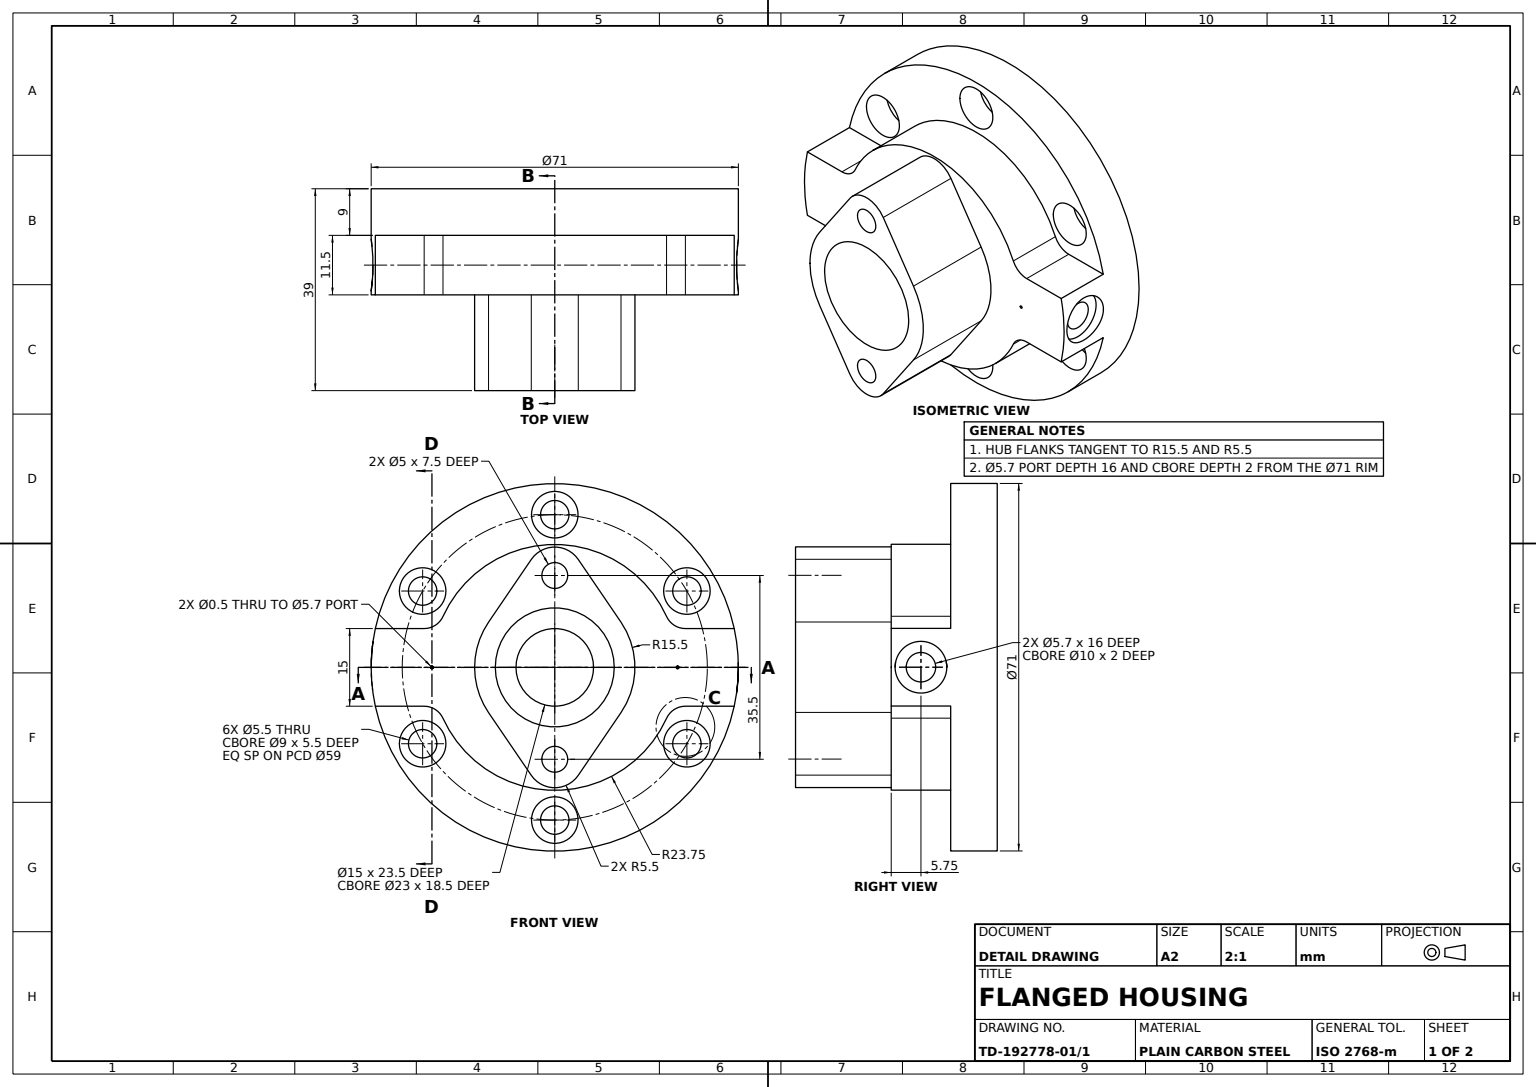
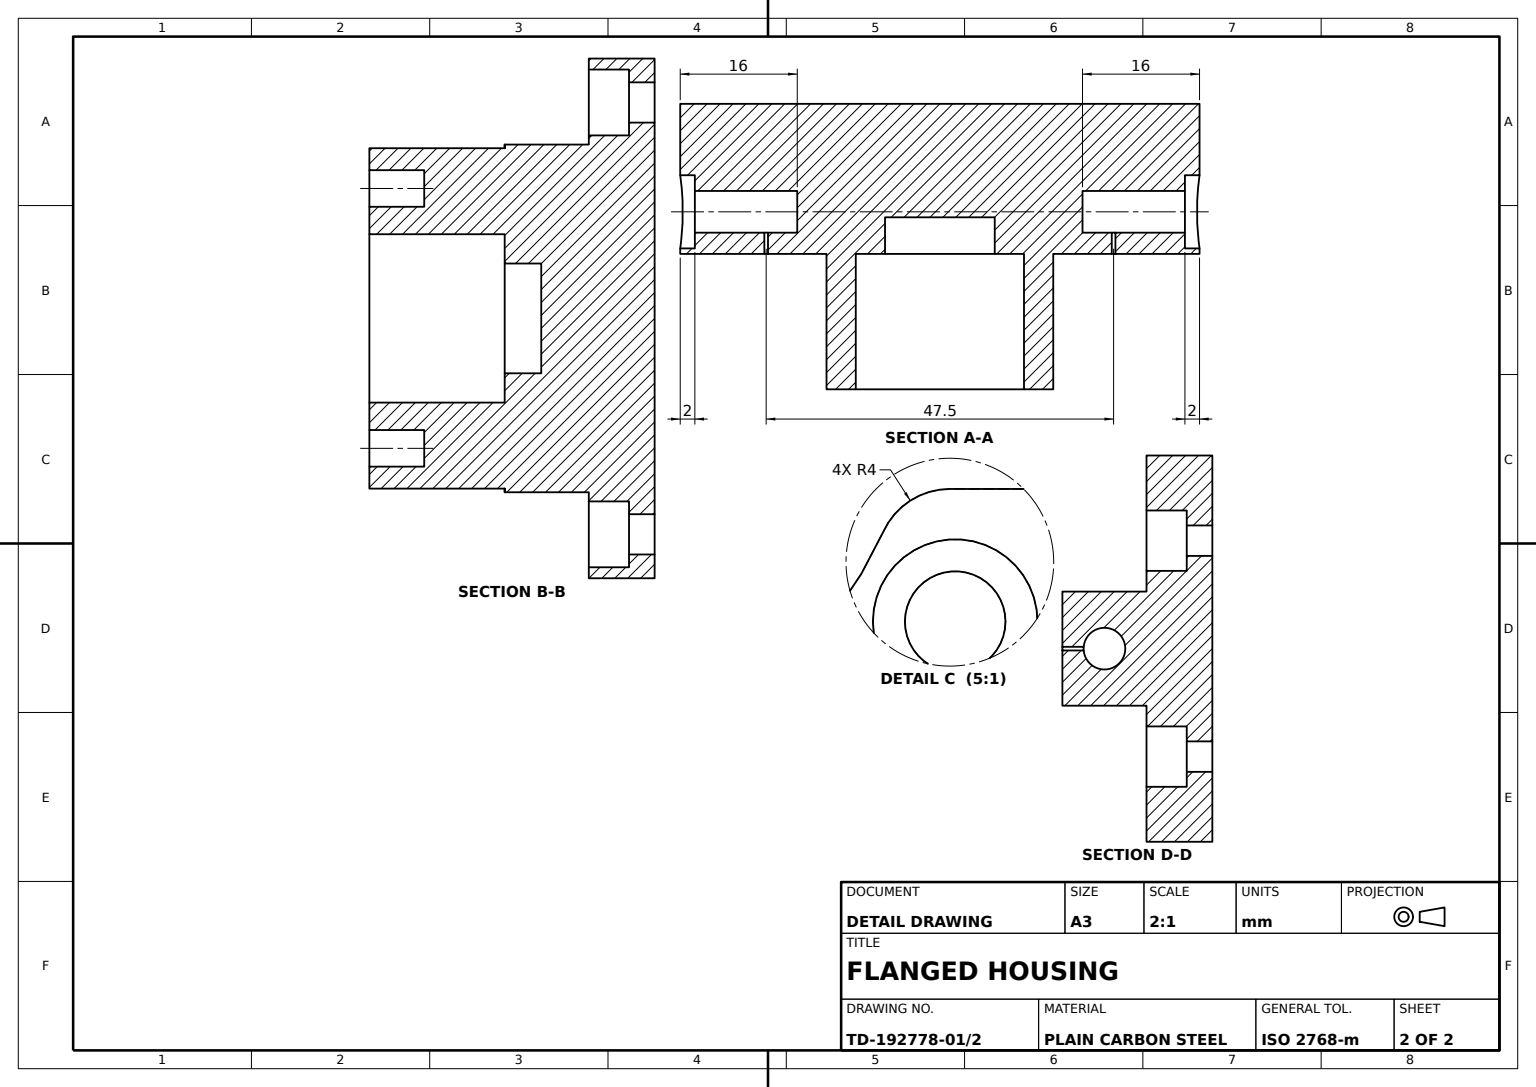
SolidWorks part; units mm, degrees
material "Plain Carbon Steel"
ref_plane "Front Plane" through (0, 0, 0) normal (0, 0, 1) x (1, 0, 0)
ref_plane "Top Plane" through (0, 0, 0) normal (0, 1, 0) x (1, 0, 0)
ref_plane "Right Plane" through (0, 0, 0) normal (1, 0, 0) x (0, 0, -1)
sketch "Flange Disc Sketch" plane through (0, 0, 0) normal (0, 0, 1) x (1, 0, 0)
  circle A0 centre (0, 0) radius 35.5
  dimension "D1" = 71
extrude "Flange Disc Ø71x9" add sketch "Flange Disc Sketch" along normal blind 9
sketch "Mounting Lug Plate Sketch" plane through (0, 0, 9) normal (0, 0, 1) x (1, 0, 0)
  line L0 (0, 0) -> (-35.5, 0) construction
  line L1 (0, 0) -> (35.5, 0) construction
  line L2 (0, 0) -> (0, 35.5) construction
  line L3 (0, 0) -> (0, -35.5) construction
  line L6 (-25.255, 7.5) -> (-34.6987, 7.5)
  line L7 (-25.255, -7.5) -> (-34.6987, -7.5)
  line L10 (25.255, 7.5) -> (34.6987, 7.5)
  line L13 (25.255, -7.5) -> (34.6987, -7.5)
  circle A1 centre (0, 0) radius 35.5 construction
  circle A2 centre (0, 0) radius 35.5
  arc A3 (-25.255, 7.5) -> (-21.6146, 9.8423) centre (-25.255, 11.5) ccw
  arc A4 (-21.6146, -9.8423) -> (-25.255, -7.5) centre (-25.255, -11.5) ccw
  arc A5 (-21.6146, -9.8423) -> (21.6146, -9.8423) centre (0, 0) ccw
  arc A6 (21.6146, 9.8423) -> (25.255, 7.5) centre (25.255, 11.5) ccw
  arc A7 (21.6146, 9.8423) -> (-21.6146, 9.8423) centre (0, 0) ccw
  arc A8 (25.255, -7.5) -> (21.6146, -9.8423) centre (25.255, -11.5) ccw
  point P21 (35.5, -7.5)
  point P23 (35.5, 7.5)
  point P37 (0, 23.75)
  circle M9 centre (0, 0) radius 35.5
  dimension "D1" = 34.6987
  dimension "D2" = 8
  dimension "D5" = 8
  dimension "D8" = 8
  dimension "D9" = 4
  dimension "D14" = 21.6146
  dimension "D17" = 25.255
  dimension "D3" = 7.5
  dimension "D4" = 9.4438
  dimension "D6" = 25.255
  dimension "D7" = 23.75
  dimension "D10" = 7.5
  dimension "D11" = 25.255
  dimension "D12" = 21.6146
  dimension "D13" = 34.6987
  dimension "D15" = 34.6987
  dimension "D16" = 7.5
  dimension "D18" = 7.5
  dimension "D19" = 21.6146
  dimension "D20" = 34.6987
extrude "Mounting Lug Plate" add sketch "Mounting Lug Plate Sketch" along normal blind 11.5 contours A8 L13 L10 A6 A7 A3 L6 L7 A4 A5 M9
sketch "Hub Profile Sketch" plane through (0, 0, 20.5) normal (0, 0, 1) x (1, 0, 0)
  line L0 (0, 0) -> (0, 23.75) construction
  line L1 (0, 0) -> (0, -23.75) construction
  line L2 (0, 23.75) -> (0, 17.75) construction
  line L3 (0, -23.75) -> (0, -17.75) construction
  line L4 (-12.8061, 8.7324) -> (-4.5441, 20.8486)
  line L5 (12.8061, 8.7324) -> (4.5441, 20.8486)
  line L6 (-12.8061, -8.7324) -> (-4.5441, -20.8486)
  line L7 (12.8061, -8.7324) -> (4.5441, -20.8486)
  arc A0 (21.6146, 9.8423) -> (-21.6146, 9.8423) centre (0, 0) ccw construction
  arc A1 (-21.6146, -9.8423) -> (21.6146, -9.8423) centre (0, 0) ccw construction
  arc A2 (-12.8061, 8.7324) -> (-12.8061, -8.7324) centre (0, 0) ccw
  arc A3 (4.5441, 20.8486) -> (-4.5441, 20.8486) centre (0, 17.75) ccw
  arc A4 (-4.5441, -20.8486) -> (4.5441, -20.8486) centre (0, -17.75) ccw
  arc A5 (12.8061, -8.7324) -> (12.8061, 8.7324) centre (0, 0) ccw
  dimension "D1" = 31
  dimension "D2" = 11
  dimension "D3" = 11
  dimension "D4" = 12.1162
  dimension "D5" = 12.1162
extrude "Hub Boss" add sketch "Hub Profile Sketch" along normal blind 18.5
ref_plane "Plane1" through (35.5, 0, 0) normal (1, 0, 0) x (0, 0, -1)
sketch "Radial Port Hole Sketch" plane through (35.5, 0, 0) normal (1, 0, 0) x (0, 0, -1)
  circle A0 centre (-14.75, 0) radius 2.85
  dimension "D1" = 5.7
  dimension "D2" = 14.75
extrude "Radial Port Hole Ø5.7" cut sketch "Radial Port Hole Sketch" against normal blind 16
sketch "Radial Port Counterbore Sketch" plane through (35.5, 0, 0) normal (1, 0, 0) x (0, 0, -1)
  circle A0 centre (-14.75, 0) radius 4.9987
  dimension "D1" = 9.9975
extrude "Radial Port Counterbore Ø10" cut sketch "Radial Port Counterbore Sketch" against normal blind 2
ref_plane "Plane2" through (0, 0, 0) normal (1, 0, 0) x (0, 0, -1)
mirror "Radial Port Mirror" about plane through (0, 0, 0) normal (1, 0, 0) of "Radial Port Counterbore Ø10", "Radial Port Hole Ø5.7"
sketch "Main Bore Sketch" plane through (0, 0, 39) normal (0, 0, 1) x (1, 0, 0)
  circle A0 centre (0, 0) radius 11.5
  dimension "D1" = 23
extrude "Main Bore Ø23" cut sketch "Main Bore Sketch" against normal blind 18.5
sketch "Through Bore Sketch" plane through (0, 0, 20.5) normal (0, 0, 1) x (1, 0, 0)
  circle A0 centre (0, 0) radius 7.5
  dimension "D1" = 15
extrude "Through Bore Ø15" cut sketch "Through Bore Sketch" against normal blind 5
sketch "Bolt Hole Sketch" plane through (0, 0, 9) normal (0, 0, 1) x (1, 0, 0)
  line L0 (0, 0) -> (0, -29.5) construction
  circle A0 centre (0, 0) radius 29.5 construction
  circle A1 centre (0, -29.5) radius 2.75
  dimension "D1" = 59
  dimension "D2" = 5.5
extrude "Bolt Hole Ø5.5" cut sketch "Bolt Hole Sketch" against normal through all
sketch "Bolt Hole Counterbore Sketch" plane through (0, 0, 9) normal (0, 0, 1) x (1, 0, 0)
  circle A0 centre (0, -29.5) radius 4.5
  dimension "D1" = 9
extrude "Bolt Hole Counterbore Ø9" cut sketch "Bolt Hole Counterbore Sketch" against normal blind 5.5
pattern_circular "Bolt Hole Pattern 6x" count 6 over 360 about axis through (0, 0, 0) along (0, 0, 1) of "Bolt Hole Counterbore Ø9", "Bolt Hole Ø5.5"
sketch "Lug Holes Sketch" plane through (0, 0, 39) normal (0, 0, 1) x (1, 0, 0)
  circle A0 centre (0, 17.75) radius 2.5
  circle A1 centre (0, -17.75) radius 2.5
  dimension "D1" = 5
  dimension "D2" = 5
extrude "Lug Holes Ø5" cut sketch "Lug Holes Sketch" against normal blind 7.5
sketch "Relief Groove Sketch" plane through (0, 0, 20.5) normal (0, 0, 1) x (1, 0, 0)
  line L0 (0, 0) -> (-23.75, 0) construction
  line L1 (0, 0) -> (23.75, 0) construction
  circle A0 centre (0, 0) radius 23.75 construction
  circle A1 centre (-23.75, 0) radius 0.25
  circle A2 centre (23.75, 0) radius 0.25
  dimension "D1" = 47.5
  dimension "D2" = 0.5
  dimension "D3" = 0.5
extrude "Relief Groove" cut sketch "Relief Groove Sketch" against normal blind 7.5
